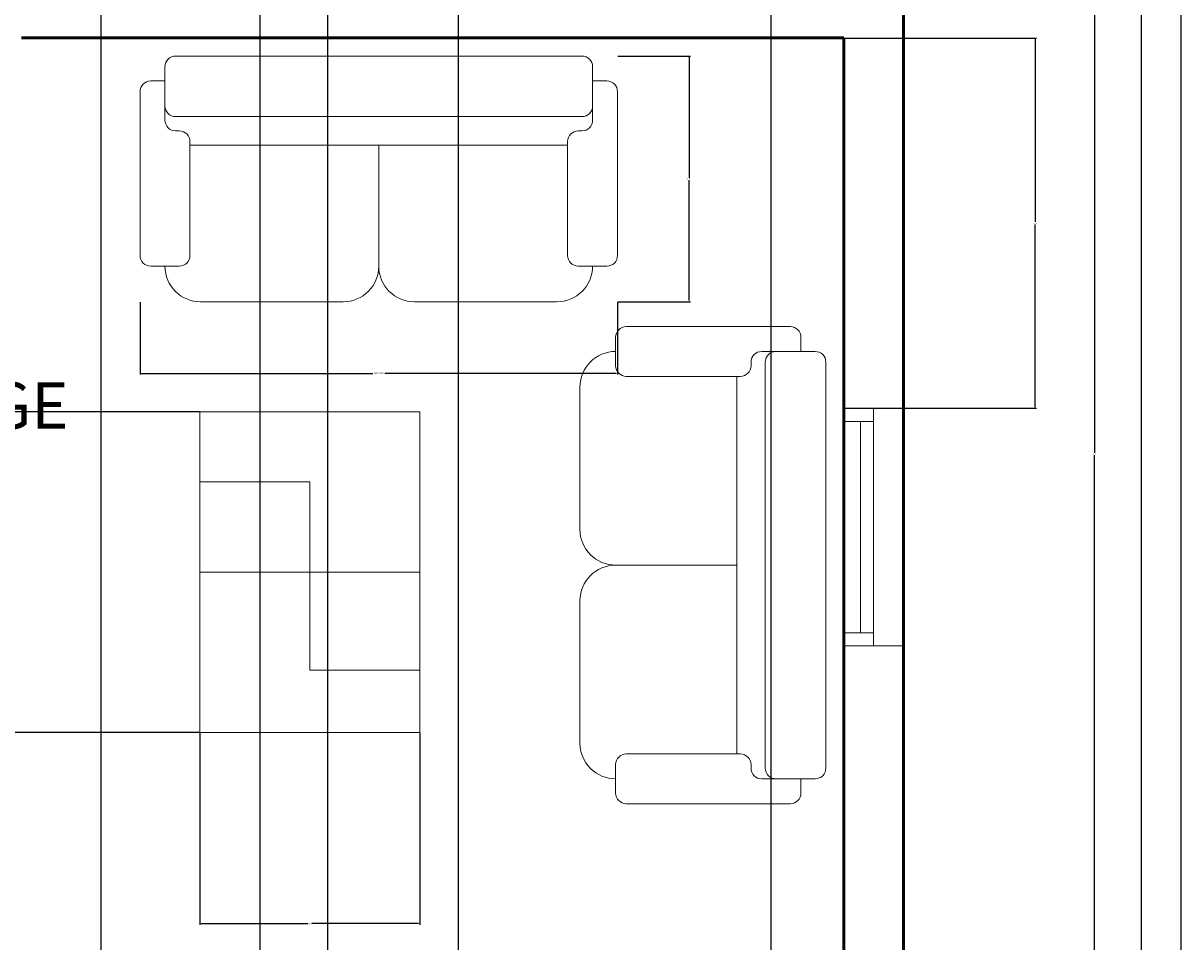
# Model space of a CAD drawing. Units: inches. Extents: x -28 to 483, y -584 to 51.
# Tile 4 of 6: x 270 to 445, y -330 to -191. Entities that reach past the tile are written whole.
import ezdxf

# ---------------------------------------------------------------- set-up
doc = ezdxf.new("R2010")
doc.units = ezdxf.units.IN
doc.header["$MEASUREMENT"] = 0
for name, color, linetype, lineweight in [('A-ANNO-DIMS', 2, 'Continuous', 18), ('A-AREA-IDEN', 7, 'Continuous', 25), ('A-FURN', 30, 'Continuous', 18), ('A-GLAZ', 5, 'Continuous', 18), ('A-WALL', 7, 'Continuous', 50), ('C-PROP', 7, 'Continuous', 25)]:
    doc.layers.add(name, color=color, linetype=linetype, lineweight=lineweight)
doc.styles.get("Standard").update_dxf_attribs({"font": 'arial.ttf'})
doc.dimstyles.get("Standard").update_dxf_attribs({"dimtxt": 0.18, "dimasz": 0.18, "dimexe": 0.18, "dimexo": 0.0625, "dimgap": 0.09, "dimtad": 0, "dimtih": 1, "dimtoh": 1, "dimdec": 4, "dimzin": 0, "dimdsep": 46, "dimtxsty": 'Standard', "dimcen": 0.09, "dimadec": 0, "dimazin": 0, "dimtfac": 1, "dimtdec": 4, "dimtofl": 0, "dimtmove": 0, "dimatfit": 3, "dimfxl": 1, "dimtolj": 1, "dimtzin": 0, "dimarcsym": 0})

# ---------------------------------------------------------------- blocks, each defined once
blk = doc.blocks.new('A$C02A636C4')
for p, q in [((1.2026, 0.6692), (0.097, 0.6692)), ((0.0679, 0.6401), (0.0679, 0.6013)), ((1.2317, 0.6401), (1.2317, 0.6013)), ((0.0679, 0.6013), (0.0291, 0.6013)), ((0.0679, 0.5334), (0.0679, 0.6013)), ((1.2317, 0.6013), (1.2705, 0.6013)), ((1.2317, 0.5334), (1.2317, 0.6013)), ((0, 0.5722), (0, 0.1261)), ((1.2996, 0.5722), (1.2996, 0.1261)), ((0.0679, 0.4946), (0.0679, 0.5431)), ((1.2317, 0.4946), (1.2317, 0.5431)), ((1.2026, 0.5043), (0.097, 0.5043)), ((0.1067, 0.4655), (0.097, 0.4655)), ((1.1929, 0.4655), (1.2026, 0.4655)), ((0.1358, 0.1261), (0.1358, 0.4364)), ((1.1638, 0.4267), (0.1358, 0.4267)), ((0.6498, 0.097), (0.6498, 0.4267)), ((1.1638, 0.1261), (1.1638, 0.4364)), ((0.0291, 0.097), (0.1067, 0.097)), ((1.2705, 0.097), (1.1929, 0.097)), ((0.1649, 0), (0.5528, 0)), ((0.7468, 0), (1.1347, 0))]:
    blk.add_line(p, q)
for centre, radius, start, end in [((0.097, 0.6401), 0.0291, 90, 180), ((1.2026, 0.6401), 0.0291, 0, 90), ((0.0291, 0.5722), 0.0291, 90, 180), ((1.2705, 0.5722), 0.0291, 0, 90), ((0.097, 0.5334), 0.0291, 180, 270), ((1.2026, 0.5334), 0.0291, 270, 0), ((0.097, 0.4946), 0.0291, 180, 270), ((1.2026, 0.4946), 0.0291, 270, 0), ((0.1067, 0.4364), 0.0291, 0, 90), ((1.1929, 0.4364), 0.0291, 90, 180), ((0.0291, 0.1261), 0.0291, 180, 270), ((0.1067, 0.1261), 0.0291, 270, 0), ((1.1929, 0.1261), 0.0291, 180, 270), ((1.2705, 0.1261), 0.0291, 270, 0), ((0.1649, 0.097), 0.097, 180, 270), ((0.5528, 0.097), 0.097, 270, 0), ((0.7468, 0.097), 0.097, 180, 270), ((1.1347, 0.097), 0.097, 270, 0)]:
    blk.add_arc(centre, radius, start, end)
blk = doc.blocks.new('WIN-36IN')
for p, q in [((0, 9), (0, 0)), ((2, 9), (2, 4.5)), ((34, 9), (34, 4.5)), ((36, 9), (36, 0)), ((34, 6.5), (2, 6.5)), ((36, 4.5), (0, 4.5))]:
    blk.add_line(p, q)
blk = doc.blocks.new('*D15')
at = {"layer": 'A-ANNO-DIMS', "color": 0, "lineweight": -2, "transparency": 16777216}
for p, q in [((287.29, -233.11), (287.29, -244.07)), ((359.57, -233.11), (359.57, -244.07)), ((287.47, -243.89), (322.52, -243.89)), ((359.39, -243.89), (324.33, -243.89))]:
    blk.add_line(p, q, dxfattribs=at)
at = {"layer": 'A-ANNO-DIMS', "color": 0, "transparency": 16777216}
for points in [[(287.47, -243.86), (287.47, -243.92), (287.29, -243.89)], [(359.39, -243.86), (359.39, -243.92), (359.57, -243.89)]]:
    blk.add_solid(points, dxfattribs=at)
at = {"layer": 'Defpoints', "color": 0, "transparency": 16777216}
for p in [(287.29, -233.05), (359.57, -233.05), (359.57, -243.89)]:
    blk.add_point(p, dxfattribs=at)
at = {"layer": 'A-ANNO-DIMS', "color": 0, "transparency": 16777216, "insert": (323.43, -243.89), "char_height": 0.18, "attachment_point": 5}
blk.add_mtext('\\A1;SOFA 72 TYP.', dxfattribs=at)
blk = doc.blocks.new('*D16')
at = {"layer": 'A-ANNO-DIMS', "color": 0, "lineweight": -2, "transparency": 16777216}
for p, q in [((359.63, -195.82), (370.6, -195.82)), ((370.42, -196), (370.42, -214.25)), ((370.42, -232.87), (370.42, -214.62)), ((359.63, -233.05), (370.6, -233.05))]:
    blk.add_line(p, q, dxfattribs=at)
at = {"layer": 'A-ANNO-DIMS', "color": 0, "transparency": 16777216}
for points in [[(370.39, -196), (370.45, -196), (370.42, -195.82)], [(370.39, -232.87), (370.45, -232.87), (370.42, -233.05)]]:
    blk.add_solid(points, dxfattribs=at)
at = {"layer": 'Defpoints', "color": 0, "transparency": 16777216}
for p in [(359.57, -195.82), (370.42, -195.82), (359.57, -233.05)]:
    blk.add_point(p, dxfattribs=at)
at = {"layer": 'A-ANNO-DIMS', "color": 0, "transparency": 16777216, "insert": (370.42, -214.43), "char_height": 0.18, "attachment_point": 5}
blk.add_mtext('\\A1;37 TYP.', dxfattribs=at)
blk = doc.blocks.new('*D22')
at = {"layer": 'A-ANNO-DIMS', "color": 0, "lineweight": -2, "transparency": 16777216}
for p, q in [((402.905662, -17.587684), (431.973162, -17.587684)), ((431.793162, -17.767684), (431.793162, -255.907684)), ((431.793162, -494.407684), (431.793162, -256.267684)), ((402.905662, -494.587684), (431.973162, -494.587684))]:
    blk.add_line(p, q, dxfattribs=at)
at = {"layer": 'A-ANNO-DIMS', "color": 0, "transparency": 16777216}
for points in [[(431.763162, -17.767684), (431.823162, -17.767684), (431.793162, -17.587684)], [(431.763162, -494.407684), (431.823162, -494.407684), (431.793162, -494.587684)]]:
    blk.add_solid(points, dxfattribs=at)
at = {"layer": 'Defpoints', "color": 0, "transparency": 16777216}
for p in [(402.843162, -17.587684), (402.843162, -494.587684), (431.793162, -494.587684)]:
    blk.add_point(p, dxfattribs=at)
at = {"layer": 'A-ANNO-DIMS', "color": 0, "transparency": 16777216, "insert": (431.793162, -256.087684), "char_height": 0.18, "attachment_point": 5}
blk.add_mtext('\\A1;477', dxfattribs=at)
blk = doc.blocks.new('*D30')
at = {"layer": 'A-ANNO-DIMS', "color": 0, "lineweight": -2, "transparency": 16777216}
for p, q in [((305.44, -116.65), (305.44, -583.72)), ((335.44, -116.65), (335.44, -583.72)), ((305.62, -583.54), (320.22, -583.54)), ((335.26, -583.54), (320.66, -583.54))]:
    blk.add_line(p, q, dxfattribs=at)
at = {"layer": 'A-ANNO-DIMS', "color": 0, "transparency": 16777216}
for points in [[(305.62, -583.51), (305.62, -583.57), (305.44, -583.54)], [(335.26, -583.51), (335.26, -583.57), (335.44, -583.54)]]:
    blk.add_solid(points, dxfattribs=at)
at = {"layer": 'Defpoints', "color": 0, "transparency": 16777216}
for p in [(305.44, -116.59), (335.44, -116.59), (335.44, -583.54)]:
    blk.add_point(p, dxfattribs=at)
at = {"layer": 'A-ANNO-DIMS', "color": 0, "transparency": 16777216, "insert": (320.44, -583.54), "char_height": 0.18, "attachment_point": 5}
blk.add_mtext('\\A1;30', dxfattribs=at)
blk = doc.blocks.new('*D31')
at = {"layer": 'A-ANNO-DIMS', "color": 0, "lineweight": -2, "transparency": 16777216}
for p, q in [((281.34, -116.65), (281.34, -583.72)), ((305.44, -116.65), (305.44, -583.72)), ((281.52, -583.54), (293.08, -583.54)), ((305.26, -583.54), (293.7, -583.54))]:
    blk.add_line(p, q, dxfattribs=at)
at = {"layer": 'A-ANNO-DIMS', "color": 0, "transparency": 16777216}
for points in [[(281.52, -583.51), (281.52, -583.57), (281.34, -583.54)], [(305.26, -583.51), (305.26, -583.57), (305.44, -583.54)]]:
    blk.add_solid(points, dxfattribs=at)
at = {"layer": 'Defpoints', "color": 0, "transparency": 16777216}
for p in [(281.34, -116.59), (305.44, -116.59), (305.44, -583.54)]:
    blk.add_point(p, dxfattribs=at)
at = {"layer": 'A-ANNO-DIMS', "color": 0, "transparency": 16777216, "insert": (293.39, -583.54), "char_height": 0.18, "attachment_point": 5}
blk.add_mtext('\\A1;24.1', dxfattribs=at)
blk = doc.blocks.new('*D35')
at = {"layer": 'A-ANNO-DIMS', "color": 0, "lineweight": -2, "transparency": 16777216}
for p, q in [((393.91, -193.09), (422.97, -193.09)), ((422.79, -193.27), (422.79, -220.95)), ((422.79, -249), (422.79, -221.32)), ((393.91, -249.18), (422.97, -249.18))]:
    blk.add_line(p, q, dxfattribs=at)
at = {"layer": 'A-ANNO-DIMS', "color": 0, "transparency": 16777216}
for points in [[(422.76, -193.27), (422.82, -193.27), (422.79, -193.09)], [(422.76, -249), (422.82, -249), (422.79, -249.18)]]:
    blk.add_solid(points, dxfattribs=at)
at = {"layer": 'Defpoints', "color": 0, "transparency": 16777216}
for p in [(393.84, -193.09), (393.84, -249.18), (422.79, -249.18)]:
    blk.add_point(p, dxfattribs=at)
at = {"layer": 'A-ANNO-DIMS', "color": 0, "transparency": 16777216, "insert": (422.79, -221.13), "char_height": 0.18, "attachment_point": 5}
blk.add_mtext('\\A1;56.09', dxfattribs=at)
blk = doc.blocks.new('*D37')
at = {"layer": 'A-ANNO-DIMS', "color": 0, "lineweight": -2, "transparency": 16777216}
for p, q in [((296.34, -298.34), (296.34, -327.41)), ((329.64, -298.34), (329.64, -327.41)), ((296.52, -327.23), (312.67, -327.23)), ((329.46, -327.23), (313.31, -327.23))]:
    blk.add_line(p, q, dxfattribs=at)
at = {"layer": 'A-ANNO-DIMS', "color": 0, "transparency": 16777216}
for points in [[(296.52, -327.2), (296.52, -327.26), (296.34, -327.23)], [(329.46, -327.2), (329.46, -327.26), (329.64, -327.23)]]:
    blk.add_solid(points, dxfattribs=at)
at = {"layer": 'Defpoints', "color": 0, "transparency": 16777216}
for p in [(296.34, -298.28), (329.64, -298.28), (296.34, -327.23)]:
    blk.add_point(p, dxfattribs=at)
at = {"layer": 'A-ANNO-DIMS', "color": 0, "transparency": 16777216, "insert": (312.99, -327.23), "char_height": 0.18, "attachment_point": 5}
blk.add_mtext('\\A1;33.3', dxfattribs=at)
blk = doc.blocks.new('*D38')
at = {"layer": 'A-ANNO-DIMS', "color": 0, "lineweight": -2, "transparency": 16777216}
for p, q in [((296.28, -249.73), (-28.29, -249.73)), ((-28.11, -249.91), (-28.11, -273.82)), ((-28.11, -298.1), (-28.11, -274.19)), ((296.28, -298.28), (-28.29, -298.28))]:
    blk.add_line(p, q, dxfattribs=at)
at = {"layer": 'A-ANNO-DIMS', "color": 0, "transparency": 16777216}
for points in [[(-28.14, -249.91), (-28.08, -249.91), (-28.11, -249.73)], [(-28.14, -298.1), (-28.08, -298.1), (-28.11, -298.28)]]:
    blk.add_solid(points, dxfattribs=at)
at = {"layer": 'Defpoints', "color": 0, "transparency": 16777216}
for p in [(296.34, -249.73), (-28.11, -298.28), (296.34, -298.28)]:
    blk.add_point(p, dxfattribs=at)
at = {"layer": 'A-ANNO-DIMS', "color": 0, "transparency": 16777216, "insert": (-28.11, -274), "char_height": 0.18, "attachment_point": 5}
blk.add_mtext('\\A1;48.54', dxfattribs=at)
blk = doc.blocks.new('*D41')
at = {"layer": 'A-ANNO-DIMS', "color": 0, "lineweight": -2, "transparency": 16777216}
for p, q in [((315.72, -337.03), (315.72, 50.54)), ((315.9, 50.36), (348.97, 50.36)), ((382.64, 50.36), (349.58, 50.36)), ((382.82, -337.03), (382.82, 50.54))]:
    blk.add_line(p, q, dxfattribs=at)
at = {"layer": 'A-ANNO-DIMS', "color": 0, "transparency": 16777216}
for points in [[(315.9, 50.39), (315.9, 50.33), (315.72, 50.36)], [(382.64, 50.39), (382.64, 50.33), (382.82, 50.36)]]:
    blk.add_solid(points, dxfattribs=at)
at = {"layer": 'Defpoints', "color": 0, "transparency": 16777216}
for p in [(382.82, 50.36), (315.72, -337.09), (382.82, -337.09)]:
    blk.add_point(p, dxfattribs=at)
at = {"layer": 'A-ANNO-DIMS', "color": 0, "transparency": 16777216, "insert": (349.27, 50.36), "char_height": 0.18, "attachment_point": 5}
blk.add_mtext('\\A1;67.1', dxfattribs=at)

msp = doc.modelspace()

# ---------------------------------------------------------------- linework, layer by layer
at = {"layer": 'A-FURN'}
for p, q in [((296.3395, -260.2958), (312.9904, -260.2958)), ((312.9904, -260.2958), (312.9904, -288.8371)), ((296.3395, -274.0046), (329.6412, -274.0046)), ((312.9904, -288.8371), (329.6412, -288.8371))]:
    msp.add_line(p, q, dxfattribs=at)
msp.add_lwpolyline([(296.3395, -249.7333), (329.6412, -249.7333), (329.6412, -298.276), (296.3395, -298.276)], close=True, dxfattribs=at)
at = {"layer": 'A-WALL'}
for p, q in [((402.8432, -17.5877), (402.8432, -494.5877)), ((269.3523, -193.0877), (393.8432, -193.0877)), ((393.8432, -193.0877), (393.8432, -332.5877))]:
    msp.add_line(p, q, dxfattribs=at)
at = {"layer": 'C-PROP'}
for p, q in [((444.8432, 21.4123), (444.8432, -554.5877)), ((438.8432, 15.4123), (438.8432, -548.5877))]:
    msp.add_line(p, q, dxfattribs=at)

# ---------------------------------------------------------------- block references
at = {"layer": 'A-FURN', "xscale": 55.62146842249675, "yscale": 55.62146842249675, "zscale": 55.62146842249675}
msp.add_blockref('A$C02A636C4', (287.2857, -233.0454), dxfattribs=at)
at = {"layer": 'A-FURN', "xscale": 55.62146842249675, "yscale": 55.62146842249675, "zscale": 55.62146842249675, "rotation": 270}
msp.add_blockref('A$C02A636C4', (353.8853, -236.7937), dxfattribs=at)
at = {"layer": 'A-GLAZ', "rotation": 89.99999999999989}
msp.add_blockref('WIN-36IN', (402.8435, -285.1794), dxfattribs=at)

# ---------------------------------------------------------------- texts
at = {"layer": 'A-AREA-IDEN', "insert": (189.5927, -245.2647), "char_height": 7, "attachment_point": 1}
msp.add_mtext_dynamic_manual_height_columns("\\pxqc;FAMILY LOUNGE\\P18'X12'", width=101.426885, gutter_width=1, heights=[0], dxfattribs=at)

# ---------------------------------------------------------------- dimensions: what is measured, and where the dimension line sits
at = {"layer": 'A-ANNO-DIMS'}
for base, p1, p2, override, picture, middle in [((382.8208, 50.3623), (315.7242, -337.0877), (382.8208, -337.0877), {"dimdec": 1, "dimlfac": 1, "dimrnd": 0, "dimzin": 0, "dimdsep": 46, "dimlunit": 2}, '*D41', (349.2725, 50.3623)), ((305.4421, -583.5377), (281.3432, -116.5877), (305.4421, -116.5877), {"dimdec": 1, "dimlfac": 1, "dimrnd": 0, "dimzin": 0, "dimdsep": 46, "dimlunit": 2}, '*D31', (293.3926, -583.5377)), ((335.4421, -583.5377), (305.4421, -116.5877), (335.4421, -116.5877), {"dimdec": 0, "dimlfac": 1, "dimrnd": 0, "dimzin": 0, "dimdsep": 46, "dimlunit": 2}, '*D30', (320.4421, -583.5377))]:
    dim = msp.add_linear_dim(base=base, p1=p1, p2=p2, dimstyle='Standard', override=override, dxfattribs=at)
    dim.commit()
    dim.dimension.update_dxf_attribs({"geometry": picture, "text_midpoint": middle})
for base, p1, p2, angle, override, picture, middle in [((431.7932, -494.5877), (402.8432, -17.5877), (402.8432, -494.5877), 270, {"dimdec": 0, "dimlfac": 1, "dimrnd": 0, "dimzin": 0, "dimdsep": 46, "dimlunit": 2}, '*D22', (431.7932, -256.0877)), ((422.7932, -249.1794), (393.8432, -193.0877), (393.8432, -249.1794), 270, {"dimdec": 2, "dimlfac": 1, "dimrnd": 0, "dimzin": 0, "dimdsep": 46, "dimlunit": 2}, '*D35', (422.7932, -221.1335)), ((-28.1068, -298.276), (296.3395, -249.7333), (296.3395, -298.276), 90, {"dimdec": 2, "dimlfac": 1, "dimrnd": 0, "dimzin": 0, "dimdsep": 46, "dimlunit": 2}, '*D38', (-28.1068, -274.0046)), ((296.3395, -327.226), (329.6412, -298.276), (296.3395, -298.276), 180, {"dimdec": 1, "dimlfac": 1, "dimrnd": 0, "dimzin": 0, "dimdsep": 46, "dimlunit": 2}, '*D37', (312.9904, -327.226))]:
    dim = msp.add_linear_dim(base=base, p1=p1, p2=p2, angle=angle, dimstyle='Standard', override=override, dxfattribs=at)
    dim.commit()
    dim.dimension.update_dxf_attribs({"geometry": picture, "text_midpoint": middle})
dim = msp.add_linear_dim(base=(370.4155, -195.8231), p1=(359.5725, -233.0454), p2=(359.5725, -195.8231), angle=90, text='<> TYP.', dimstyle='Standard', override={"dimdec": 0, "dimlfac": 1, "dimrnd": 0, "dimzin": 0, "dimdsep": 46, "dimlunit": 2}, dxfattribs=at)
dim.commit()
dim.dimension.update_dxf_attribs({"geometry": '*D16', "text_midpoint": (370.4155, -214.4343)})
dim = msp.add_linear_dim(base=(359.5725, -243.8884), p1=(287.2857, -233.0454), p2=(359.5725, -233.0454), text='SOFA <> TYP.', dimstyle='Standard', override={"dimdec": 0, "dimlfac": 1, "dimrnd": 0, "dimzin": 0, "dimdsep": 46, "dimlunit": 2}, dxfattribs=at)
dim.commit()
dim.dimension.update_dxf_attribs({"geometry": '*D15', "text_midpoint": (323.4291, -243.8884)})

doc.saveas('drawing.dxf')
